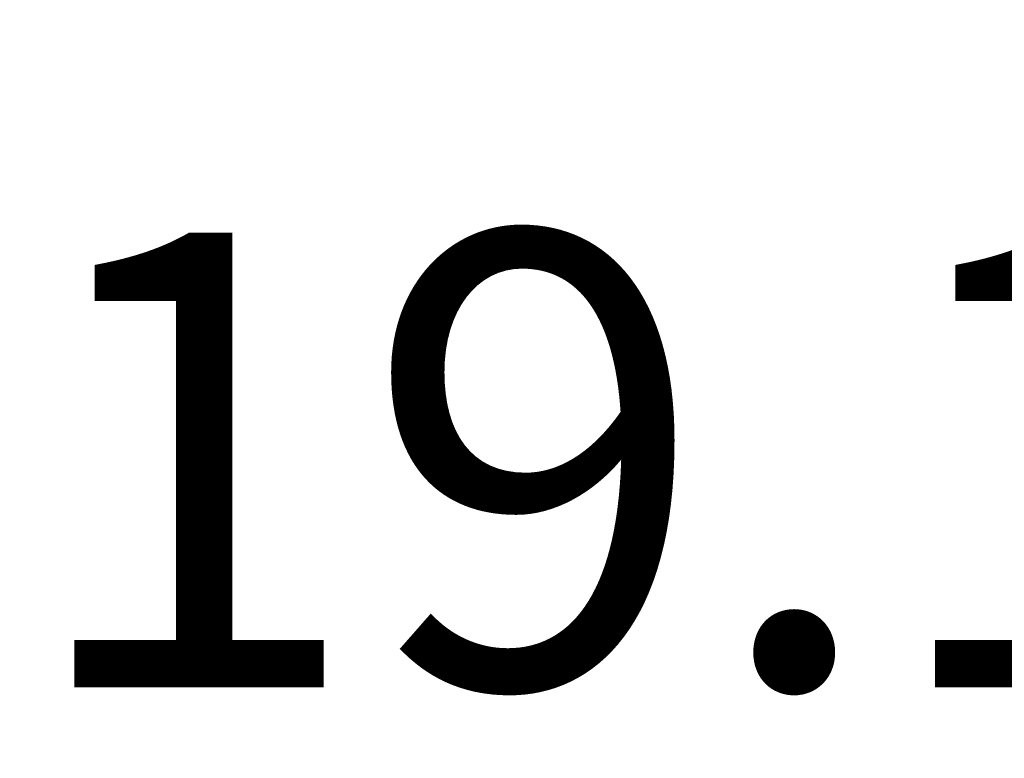
# Model space of a CAD drawing. Units: inches. Extents: x 305 to 776, y 38 to 479.
# Tile 2 of 14: x 305 to 349, y 218 to 250. Entities that reach past the tile are written whole.
import ezdxf

# ---------------------------------------------------------------- set-up
doc = ezdxf.new("R2010")
doc.units = ezdxf.units.IN
doc.header["$MEASUREMENT"] = 0
doc.layers.add('A-ANNO-DIMS', color=2, linetype='Continuous', lineweight=18)
doc.styles.get("Standard").update_dxf_attribs({"font": 'arial.ttf'})
doc.dimstyles.get("Standard").update_dxf_attribs({"dimtxt": 20, "dimasz": 0.18, "dimexe": 0.18, "dimexo": 0.0625, "dimgap": 0.09, "dimtad": 0, "dimtih": 1, "dimtoh": 1, "dimdec": 4, "dimzin": 0, "dimdsep": 46, "dimtxsty": 'Standard', "dimcen": 0.09, "dimadec": 0, "dimazin": 0, "dimtfac": 1, "dimtdec": 4, "dimtofl": 0, "dimtmove": 0, "dimatfit": 3, "dimfxl": 1, "dimtolj": 1, "dimtzin": 0, "dimarcsym": 0})

# ---------------------------------------------------------------- blocks, each defined once
blk = doc.blocks.new('*D74')
at = {"layer": 'A-ANNO-DIMS', "color": 0, "lineweight": -2, "transparency": 16777216}
for p, q in [((399.57, 250.482), (372.451, 250.482)), ((372.631, 250.302), (372.631, 231.472)), ((404.07, 231.292), (372.451, 231.292)), ((372.631, 231.112), (372.451, 231.112)), ((372.631, 231.292), (372.631, 231.112))]:
    blk.add_line(p, q, dxfattribs=at)
at = {"layer": 'A-ANNO-DIMS', "color": 0, "transparency": 16777216}
for points in [[(372.601, 250.302), (372.661, 250.302), (372.631, 250.482)], [(372.601, 231.472), (372.661, 231.472), (372.631, 231.292)]]:
    blk.add_solid(points, dxfattribs=at)
at = {"layer": 'Defpoints', "color": 0, "transparency": 16777216}
for p in [(399.633, 250.482), (372.631, 231.292), (404.133, 231.292)]:
    blk.add_point(p, dxfattribs=at)
at = {"layer": 'A-ANNO-DIMS', "color": 0, "transparency": 16777216, "insert": (339.537, 231.112), "char_height": 20, "attachment_point": 5}
blk.add_mtext('\\A1;19.19', dxfattribs=at)

msp = doc.modelspace()

# ---------------------------------------------------------------- dimensions: what is measured, and where the dimension line sits
at = {"layer": 'A-ANNO-DIMS'}
dim = msp.add_linear_dim(base=(372.6314, 231.2915), p1=(399.6329, 250.4819), p2=(404.1329, 231.2915), angle=90, dimstyle='Standard', override={"dimdec": 2, "dimlfac": 1, "dimrnd": 0, "dimzin": 0, "dimdsep": 46, "dimlunit": 2}, dxfattribs=at)
dim.commit()
dim.dimension.update_dxf_attribs({"geometry": '*D74', "text_midpoint": (339.5374, 231.1115)})

doc.saveas('drawing.dxf')
